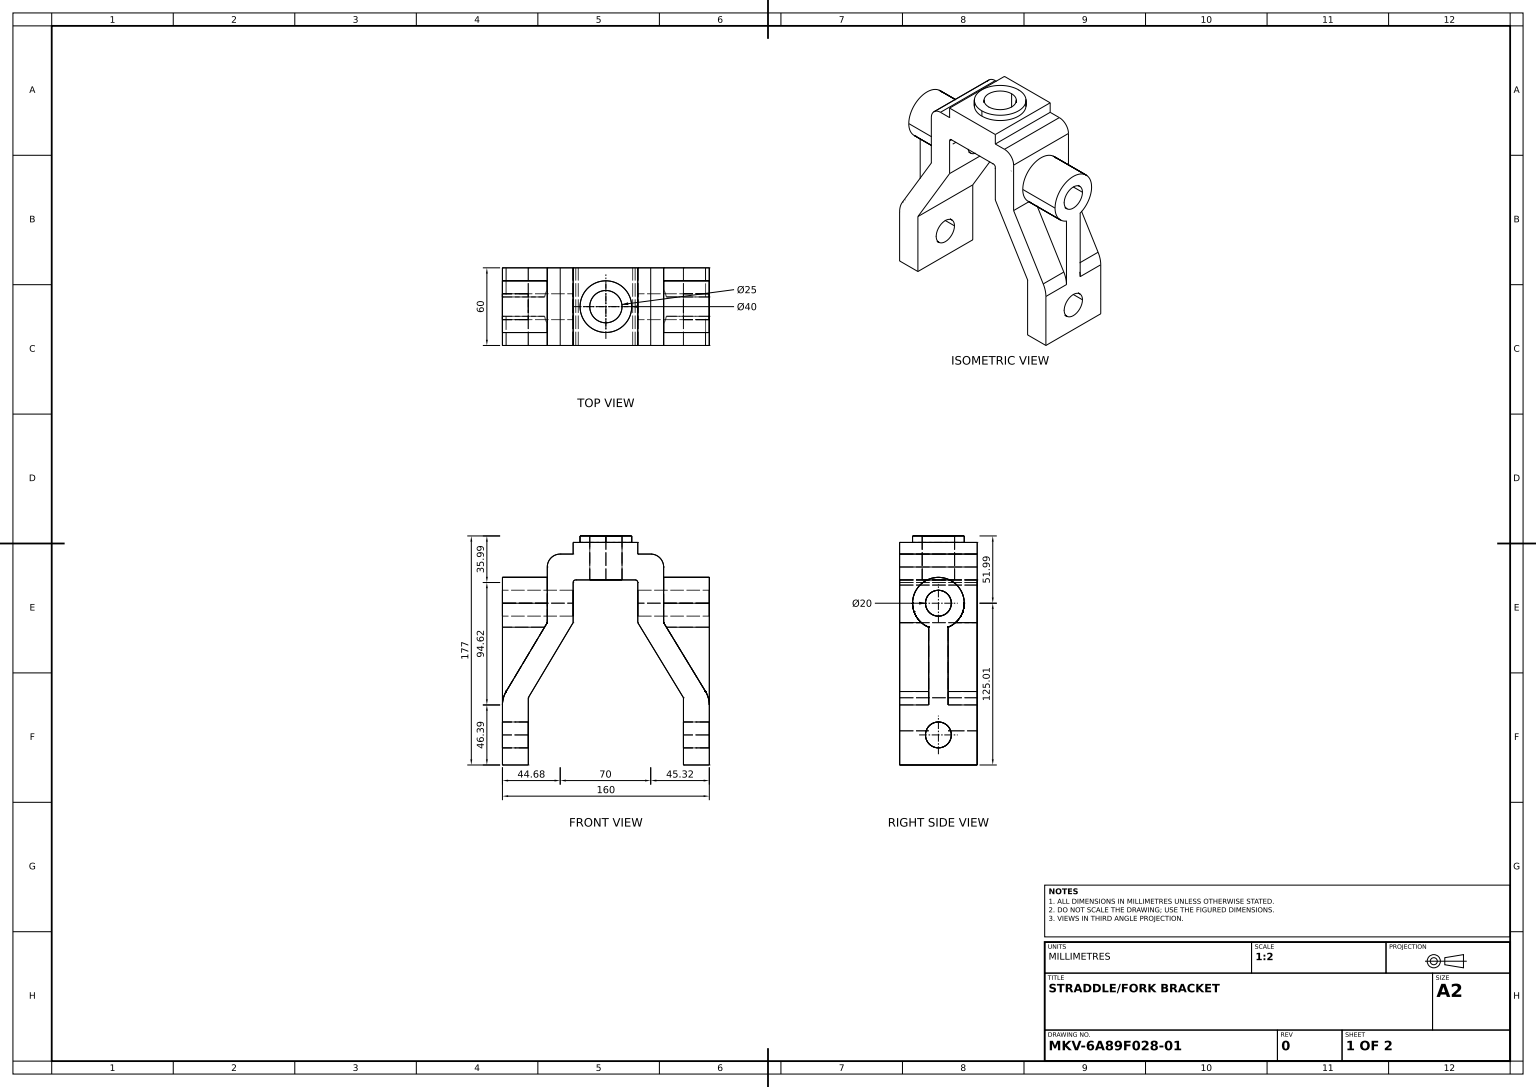
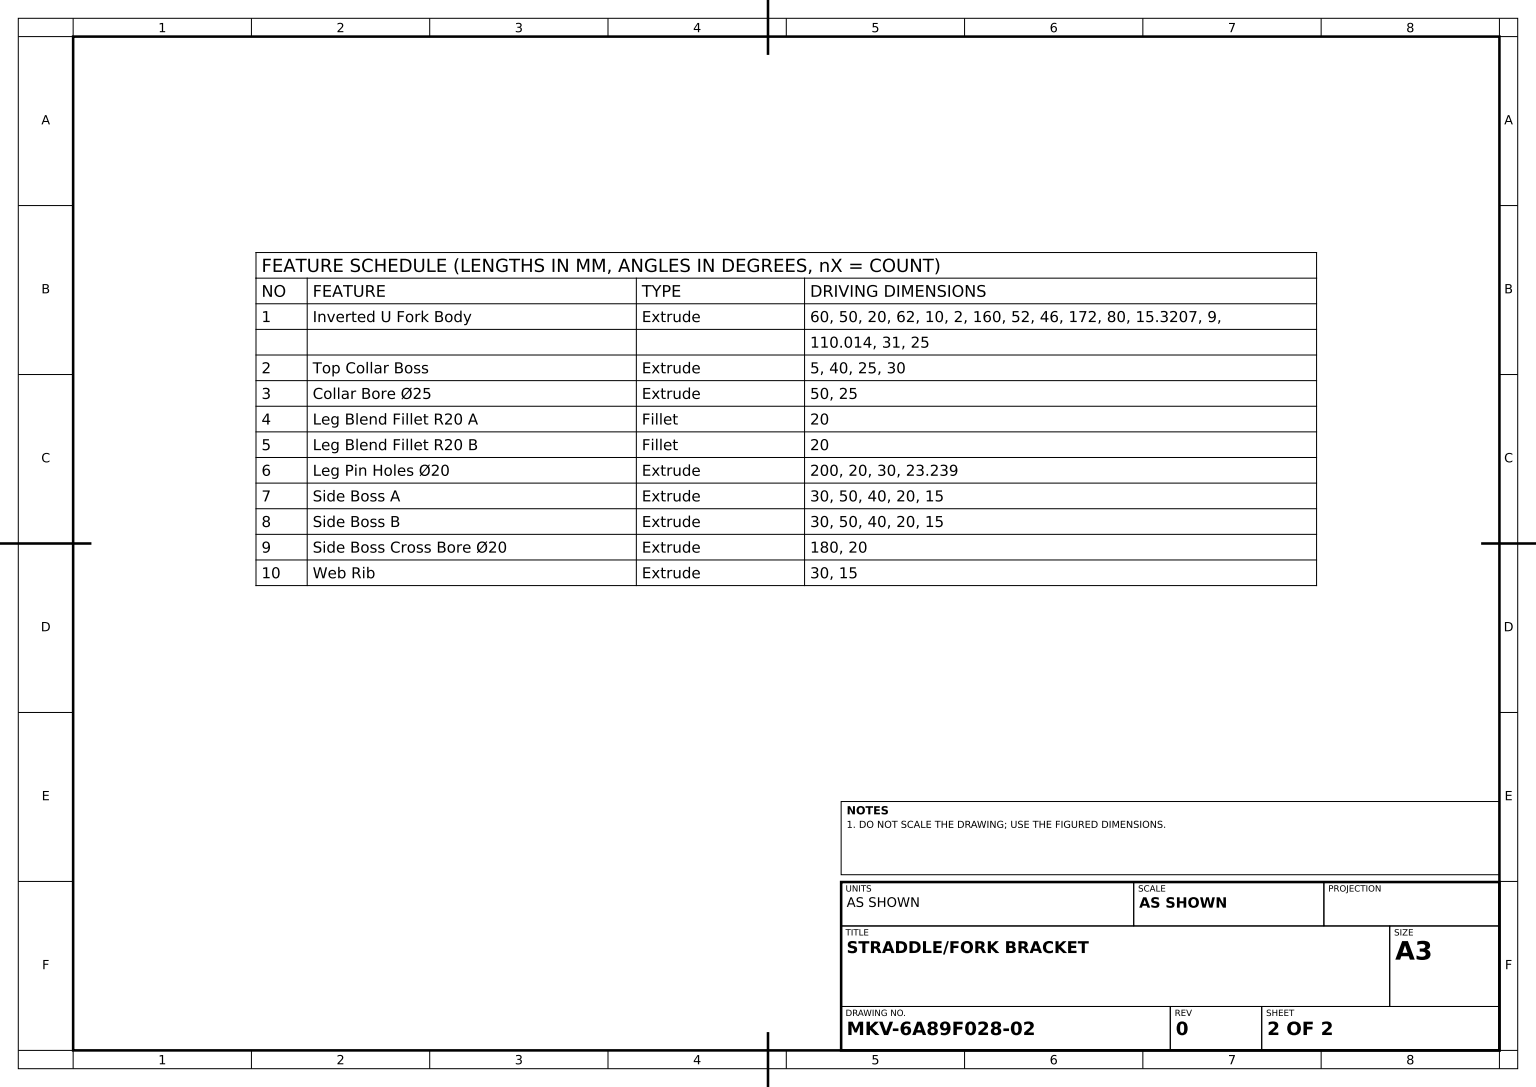
SolidWorks part; units mm, degrees
material "Plain Carbon Steel"
ref_plane "Front Plane" through (0, 0, 0) normal (0, 0, 1) x (1, 0, 0)
ref_plane "Top Plane" through (0, 0, 0) normal (0, 1, 0) x (1, 0, 0)
ref_plane "Right Plane" through (0, 0, 0) normal (1, 0, 0) x (0, 0, -1)
sketch "Fork Profile Sketch" plane through (0, 0, 0) normal (0, 0, 1) x (1, 0, 0)
  line L1 (80, 0) -> (60, 0)
  line L2 (-80, 0) -> (-60, 0)
  line L3 (-25.3207, 110.0135) -> (-25.3207, 141.0135)
  line L5 (-60, 0) -> (-60, 52)
  line L7 (60, 0) -> (60, 52)
  line L9 (60, 52) -> (24.6793, 110.0135)
  line L10 (-80, 0) -> (-80, 52)
  line L12 (-80, 52) -> (-45.3207, 110.0135)
  line L14 (-60, 52) -> (-25.3207, 110.0135)
  line L15 (-10, 172) -> (10, 172)
  line L16 (10, 172) -> (24.6793, 172)
  line L17 (-10, 172) -> (-25.3207, 172)
  line L18 (-45.3207, 110.0135) -> (-45.3207, 153)
  line L19 (-35.3207, 163) -> (-25.3207, 163)
  line L20 (-25.3207, 163) -> (-25.3207, 172)
  line L21 (24.6793, 172) -> (24.6793, 163)
  line L22 (24.6793, 163) -> (34.6793, 163)
  line L23 (44.6793, 153) -> (44.6793, 110.0135)
  line L24 (-23.3207, 143.0135) -> (22.6793, 143.0135)
  line L25 (24.6793, 141.0135) -> (24.6793, 110.0135)
  line L26 (-80, 0) -> (-60, 0)
  line L27 (80, 0) -> (80, 52)
  line L28 (80, 52) -> (44.6793, 110.0135)
  line L29 (60, 0) -> (80, 0)
  arc A0 (34.6793, 163) -> (44.6793, 153) centre (34.6793, 153) cw
  arc A1 (-45.3207, 153) -> (-35.3207, 163) centre (-35.3207, 153) cw
  arc A2 (22.6793, 143.0135) -> (24.6793, 141.0135) centre (22.6793, 141.0135) cw
  arc A3 (-25.3207, 141.0135) -> (-23.3207, 143.0135) centre (-23.3207, 141.0135) cw
  point P4 (0, 0)
  point P15 (-0.3207, 110)
  point P21 (0, 172)
  point P37 (0, 0)
  dimension "D9" = 10
  dimension "D1" = 2
  dimension "D2" = 52
  dimension "D3" = 160
  dimension "D4" = 50
  dimension "D5" = 20
  dimension "D6" = 20
  dimension "D7" = 50
  dimension "D8" = 62
  dimension "D10" = 52
  dimension "D11" = 46
  dimension "D12" = 172
  dimension "D13" = 20
  dimension "D14" = 80
  dimension "D15" = 20
  dimension "D16" = 15.3207
  dimension "D17" = 9
  dimension "D18" = 110.0135
  dimension "D19" = 31
  dimension "D20" = 25
extrude "Inverted U Fork Body" add sketch "Fork Profile Sketch" along normal blind 60 contours L3 A3 L24 A2 L25 L9 L7 L1 L27 L28 L23 A0 L22 L21 L16 L15 L17 L20 L19 A1 L18 L12 L10 L2 L5 L14
sketch "Top Collar Boss Sketch" plane through (0, 172, 0) normal (0, 1, 0) x (1, 0, 0)
  line L0 (-25.3207, -60) -> (24.6793, -60) construction
  circle A0 centre (0, -30) radius 20
  circle A1 centre (0, -30) radius 12.5
  dimension "D1" = 40
  dimension "D2" = 25
  dimension "D3" = 30
  dimension "D4" = 30
extrude "Top Collar Boss" add sketch "Top Collar Boss Sketch" along normal blind 5
sketch "Collar Bore Sketch" plane through (0, 172, 0) normal (0, 1, 0) x (1, 0, 0)
  circle A0 centre (0, -30) radius 12.5
  dimension "D1" = 25
extrude "Collar Bore Ø25" cut sketch "Collar Bore Sketch" against normal blind 50
fillet "Leg Blend Fillet R20 A" radius 20 1 edges at (-80, 52, 30)
fillet "Leg Blend Fillet R20 B" radius 20 1 edges at (80, 52, 30)
sketch "Leg Pin Hole Sketch" plane through (-80, 0, 0) normal (-1, 0, 0) x (0, 0, 1)
  line L0 (60, 0) -> (60, 46.4779) construction
  line L1 (60, 46.4779) -> (0, 46.4779) construction
  circle A0 centre (30, 23.239) radius 10
  dimension "D1" = 20
  dimension "D2" = 30
  dimension "D3" = 23.239
extrude "Leg Pin Holes Ø20" cut sketch "Leg Pin Hole Sketch" against normal blind 200
ref_plane "Side Boss A Plane" through (30, 0, 0) normal (1, 0, 0) x (0, 0, -1)
sketch "Side Boss A Sketch" plane through (30, 0, 0) normal (1, 0, 0) x (0, 0, -1)
  line L0 (-60, 110.0135) -> (0, 110.0135) construction
  line L2 (0, 153) -> (0, 110.0135) construction
  circle A0 centre (-30, 125.0135) radius 20
  circle A1 centre (-30, 125.0135) radius 10
  dimension "D1" = 40
  dimension "D2" = 20
  dimension "D3" = 15
  dimension "D4" = 30
extrude "Side Boss A" add sketch "Side Boss A Sketch" along normal blind 50
ref_plane "Side Boss B Plane" through (-30, 0, 0) normal (1, 0, 0) x (0, 0, -1)
sketch "Side Boss B Sketch" plane through (-30, 0, 0) normal (1, 0, 0) x (0, 0, -1)
  line L0 (-60, 110.0135) -> (0, 110.0135) construction
  line L1 (-60, 110.0135) -> (-60, 153) construction
  circle A0 centre (-30, 125.0135) radius 20
  circle A1 centre (-30, 125.0135) radius 10
  dimension "D1" = 40
  dimension "D2" = 20
  dimension "D3" = 15
  dimension "D4" = 30
extrude "Side Boss B" add sketch "Side Boss B Sketch" against normal blind 50
sketch "Side Boss Cross Bore Sketch" plane through (44.6793, 0, 0) normal (1, 0, 0) x (0, 0, -1)
  circle A0 centre (-30, 125.0135) radius 10
  dimension "D1" = 20
extrude "Side Boss Cross Bore Ø20" cut sketch "Side Boss Cross Bore Sketch" against normal blind 180
ref_plane "Web Rib Plane" through (0, 0, 30) normal (0, 0, 1) x (1, 0, 0)
sketch "Web Rib Sketch" plane through (0, 0, 30) normal (0, 0, 1) x (1, 0, 0)
  line L0 (-45.3207, 110.0135) -> (-80, 110.0135)
  line L1 (-80, 145.0135) -> (-80, 105.0135) construction
  line L2 (-80, 110.0135) -> (-80, 46.4779)
  line L3 (-80, 46.4779) -> (-45.3207, 110.0135)
  line L4 (44.6793, 110.0135) -> (80, 110.0135)
  line L5 (80, 105.0135) -> (80, 145.0135) construction
  line L6 (80, 110.0135) -> (80, 46.3906)
  line L7 (80, 46.3906) -> (44.6793, 110.0135)
extrude "Web Rib" add sketch "Web Rib Sketch" along normal mid plane 15
